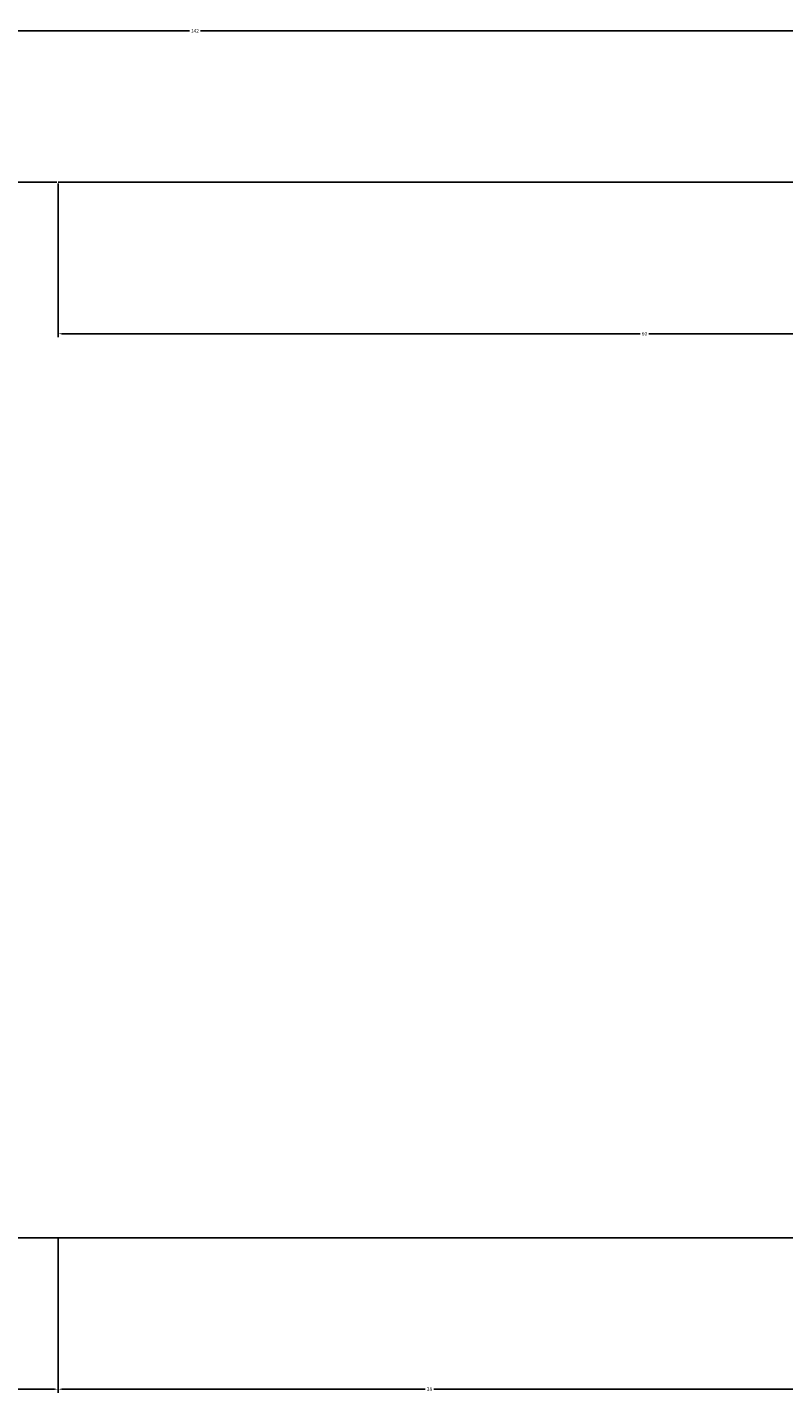
# Model space of a CAD drawing. Units: millimetres. Extents: x 223 to 381, y -8 to 62.
# Tile 2 of 5: x 293 to 332, y -8 to 62. Entities that reach past the tile are written whole.
import ezdxf

# ---------------------------------------------------------------- set-up
doc = ezdxf.new("R2010")
doc.units = ezdxf.units.MM
doc.layers.add('M-CONS', color=8, linetype='Continuous', lineweight=13)
doc.layers.add('M-DIMS', color=2, linetype='Continuous', lineweight=18)
doc.styles.get("Standard").update_dxf_attribs({"font": 'arial.ttf'})
doc.dimstyles.get("Standard").update_dxf_attribs({"dimtxt": 0.18, "dimasz": 0.18, "dimexe": 0.18, "dimexo": 0.0625, "dimgap": 0.09, "dimtad": 0, "dimtih": 1, "dimtoh": 1, "dimdec": 4, "dimzin": 0, "dimdsep": 46, "dimtxsty": 'Standard', "dimcen": 0.09, "dimadec": 0, "dimazin": 0, "dimtfac": 1, "dimtdec": 4, "dimtofl": 0, "dimtmove": 0, "dimatfit": 3, "dimfxl": 1, "dimtolj": 1, "dimtzin": 0, "dimarcsym": 0})

# ---------------------------------------------------------------- blocks, each defined once
blk = doc.blocks.new('*D1')
at = {"layer": 'Defpoints', "color": 0, "transparency": 16777216}
for p in [(372.659, 61.75), (372.659, 27), (230.659, 0)]:
    blk.add_point(p, dxfattribs=at)
at = {"layer": 'M-DIMS', "color": 0, "lineweight": -2, "transparency": 16777216}
for p, q in [((230.659, 0.062), (230.659, 61.93)), ((230.839, 61.75), (301.38, 61.75)), ((372.479, 61.75), (301.939, 61.75)), ((372.659, 27.062), (372.659, 61.93))]:
    blk.add_line(p, q, dxfattribs=at)
at = {"layer": 'M-DIMS', "color": 0, "transparency": 16777216}
for points in [[(230.839, 61.78), (230.839, 61.72), (230.659, 61.75)], [(372.479, 61.78), (372.479, 61.72), (372.659, 61.75)]]:
    blk.add_solid(points, dxfattribs=at)
at = {"layer": 'M-DIMS', "color": 0, "transparency": 16777216, "insert": (301.659, 61.75), "char_height": 0.18, "attachment_point": 5}
blk.add_mtext('\\A1;142', dxfattribs=at)
blk = doc.blocks.new('*D5')
at = {"layer": 'Defpoints', "color": 0, "transparency": 16777216}
for p in [(285.376, 0), (294.659, 0), (294.659, -7.75)]:
    blk.add_point(p, dxfattribs=at)
at = {"layer": 'M-DIMS', "color": 0, "lineweight": -2, "transparency": 16777216}
for p, q in [((285.376, -0.062), (285.376, -7.93)), ((294.659, -0.062), (294.659, -7.93)), ((285.556, -7.75), (289.624, -7.75)), ((294.479, -7.75), (290.411, -7.75))]:
    blk.add_line(p, q, dxfattribs=at)
at = {"layer": 'M-DIMS', "color": 0, "transparency": 16777216}
for points in [[(285.556, -7.72), (285.556, -7.78), (285.376, -7.75)], [(294.479, -7.72), (294.479, -7.78), (294.659, -7.75)]]:
    blk.add_solid(points, dxfattribs=at)
at = {"layer": 'M-DIMS', "color": 0, "transparency": 16777216, "insert": (290.018, -7.75), "char_height": 0.18, "attachment_point": 5}
blk.add_mtext('\\A1;9.283', dxfattribs=at)
blk = doc.blocks.new('*D6')
at = {"layer": 'Defpoints', "color": 0, "transparency": 16777216}
for p in [(294.659, 0), (332.659, 0), (332.659, -7.75)]:
    blk.add_point(p, dxfattribs=at)
at = {"layer": 'M-DIMS', "color": 0, "lineweight": -2, "transparency": 16777216}
for p, q in [((294.659, -0.062), (294.659, -7.93)), ((332.659, -0.062), (332.659, -7.93)), ((294.839, -7.75), (313.44, -7.75)), ((332.479, -7.75), (313.878, -7.75))]:
    blk.add_line(p, q, dxfattribs=at)
at = {"layer": 'M-DIMS', "color": 0, "transparency": 16777216}
for points in [[(294.839, -7.72), (294.839, -7.78), (294.659, -7.75)], [(332.479, -7.72), (332.479, -7.78), (332.659, -7.75)]]:
    blk.add_solid(points, dxfattribs=at)
at = {"layer": 'M-DIMS', "color": 0, "transparency": 16777216, "insert": (313.659, -7.75), "char_height": 0.18, "attachment_point": 5}
blk.add_mtext('\\A1;38', dxfattribs=at)
blk = doc.blocks.new('*D7')
at = {"layer": 'Defpoints', "color": 0, "transparency": 16777216}
for p in [(294.659, 54), (354.659, 54), (294.659, 46.25)]:
    blk.add_point(p, dxfattribs=at)
at = {"layer": 'M-DIMS', "color": 0, "lineweight": -2, "transparency": 16777216}
for p, q in [((294.659, 53.938), (294.659, 46.07)), ((354.659, 53.938), (354.659, 46.07)), ((294.839, 46.25), (324.44, 46.25)), ((354.479, 46.25), (324.878, 46.25))]:
    blk.add_line(p, q, dxfattribs=at)
at = {"layer": 'M-DIMS', "color": 0, "transparency": 16777216}
for points in [[(294.839, 46.28), (294.839, 46.22), (294.659, 46.25)], [(354.479, 46.28), (354.479, 46.22), (354.659, 46.25)]]:
    blk.add_solid(points, dxfattribs=at)
at = {"layer": 'M-DIMS', "color": 0, "transparency": 16777216, "insert": (324.659, 46.25), "char_height": 0.18, "attachment_point": 5}
blk.add_mtext('\\A1;60', dxfattribs=at)
blk = doc.blocks.new('*D11')
at = {"layer": 'Defpoints', "color": 0, "transparency": 16777216}
for p in [(222.909, 54), (294.659, 54), (230.659, 0)]:
    blk.add_point(p, dxfattribs=at)
at = {"layer": 'M-DIMS', "color": 0, "lineweight": -2, "transparency": 16777216}
for p, q in [((294.597, 54), (222.729, 54)), ((222.909, 53.82), (222.909, 27.182)), ((222.909, 0.18), (222.909, 26.818)), ((230.597, 0), (222.729, 0))]:
    blk.add_line(p, q, dxfattribs=at)
at = {"layer": 'M-DIMS', "color": 0, "transparency": 16777216}
for points in [[(222.879, 53.82), (222.939, 53.82), (222.909, 54)], [(222.879, 0.18), (222.939, 0.18), (222.909, 0)]]:
    blk.add_solid(points, dxfattribs=at)
at = {"layer": 'M-DIMS', "color": 0, "transparency": 16777216, "insert": (222.909, 27), "char_height": 0.18, "attachment_point": 5}
blk.add_mtext('\\A1;54', dxfattribs=at)

msp = doc.modelspace()

# ---------------------------------------------------------------- linework, layer by layer
at = {"layer": 'M-CONS', "extrusion": (0, -1, 0)}
for p, q in [((260.6592, 0, 97.6363), (332.6592, 0, 97.6363)), ((294.6592, 0, 50.3189), (285.3762, 0, 50.6343)), ((354.6592, 0, 85.6363), (294.6592, 0, 85.6363)), ((294.6592, 0, 85.6363), (294.6592, 0, 50.3189))]:
    msp.add_line(p, q, dxfattribs=at)
at = {"layer": 'M-CONS', "extrusion": (0, -1, 0), "elevation": -54}
msp.add_lwpolyline([(294.6592, 85.6363), (354.6592, 85.6363), (354.6592, 63.6363), (294.6592, 63.6363)], close=True, dxfattribs=at)

# ---------------------------------------------------------------- dimensions: what is measured, and where the dimension line sits
at = {"layer": 'M-DIMS'}
for base, p1, p2, override, picture, middle in [((372.6592, 61.75), (230.6592, 0), (372.6592, 27), {"dimdec": 0, "dimlfac": 1, "dimrnd": 0, "dimzin": 0, "dimdsep": 46, "dimlunit": 2}, '*D1', (301.6592, 61.75)), ((294.6592, -7.75), (285.3762, 0), (294.6592, 0), {"dimdec": 3, "dimlfac": 1, "dimrnd": 0, "dimzin": 0, "dimdsep": 46, "dimlunit": 2}, '*D5', (290.0177, -7.75)), ((332.6592, -7.75), (294.6592, 0), (332.6592, 0), {"dimdec": 0, "dimlfac": 1, "dimrnd": 0, "dimzin": 0, "dimdsep": 46, "dimlunit": 2}, '*D6', (313.6592, -7.75))]:
    dim = msp.add_linear_dim(base=base, p1=p1, p2=p2, dimstyle='Standard', override=override, dxfattribs=at)
    dim.commit()
    dim.dimension.update_dxf_attribs({"geometry": picture, "text_midpoint": middle})
for base, p1, angle, picture, middle in [((222.9092, 54), (230.6592, 0), 90, '*D11', (222.9092, 27)), ((294.6592, 46.25), (354.6592, 54), 180, '*D7', (324.6592, 46.25))]:
    dim = msp.add_linear_dim(base=base, p1=p1, p2=(294.6592, 54), angle=angle, dimstyle='Standard', override={"dimdec": 0, "dimlfac": 1, "dimrnd": 0, "dimzin": 0, "dimdsep": 46, "dimlunit": 2}, dxfattribs=at)
    dim.commit()
    dim.dimension.update_dxf_attribs({"geometry": picture, "text_midpoint": middle})

doc.saveas('drawing.dxf')
